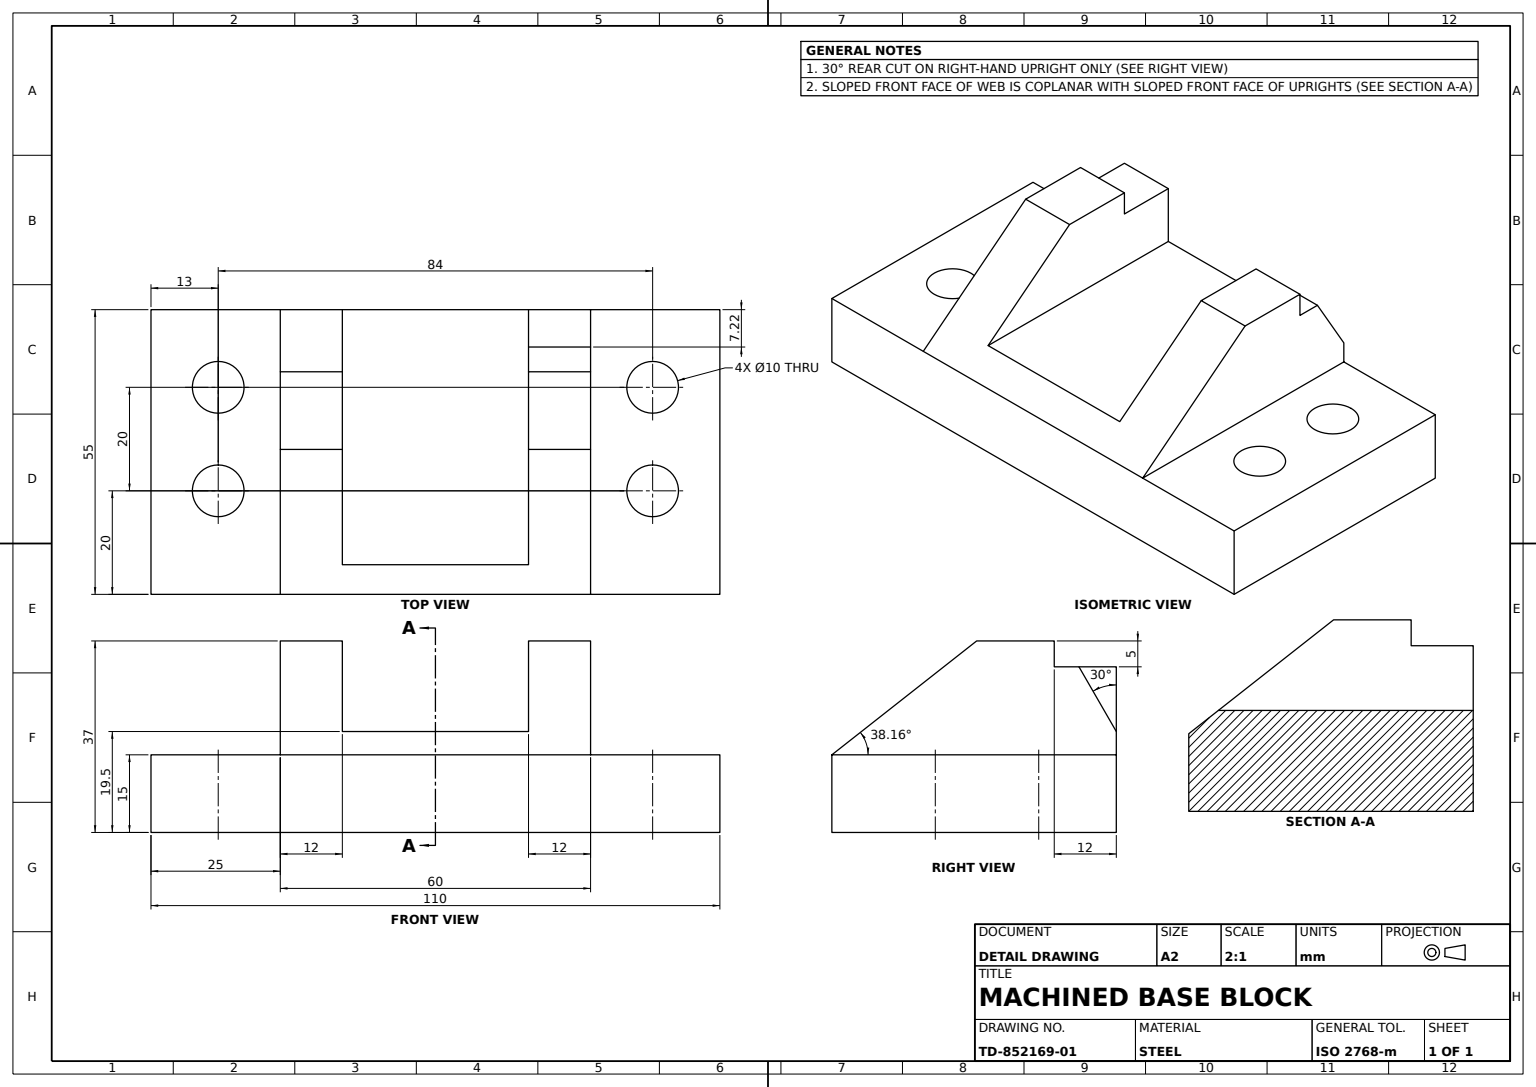
from build123d import *

# Parameters (mm, degrees)
BASE_PLATE_SKETCH_W    = 110
BASE_PLATE_SKETCH_H    = 55
BASE_PLATE_SKETCH_R    = 5
BASE_PLATE_DEPTH       = 15
V_BLOCK_UPRIGHTS_DEPTH = 55
UPRIGHT_NOTCH_SKETCH_W = 12
UPRIGHT_NOTCH_SKETCH_H = 5
UPRIGHT_NOTCH_DEPTH    = 108.791465339
ANGLED_CUT_30DEG_DEPTH = 12


with BuildPart() as part:
    # Base Plate Sketch → Base Plate (new body)
    with BuildSketch(Plane(origin=(0, 0, 0), x_dir=(1, 0, 0), z_dir=(0, 1, 0))):
        with Locations((0, 27.5)):
            Rectangle(BASE_PLATE_SKETCH_W, BASE_PLATE_SKETCH_H)
        with Locations(Location((-42, 40, 0), (0, 0, 270))):
            Circle(BASE_PLATE_SKETCH_R, mode=Mode.SUBTRACT)
        with Locations(Location((-42, 20, 0), (0, 0, 270))):
            Circle(BASE_PLATE_SKETCH_R, mode=Mode.SUBTRACT)
        with Locations(Location((42, 20, 0), (0, 0, 90))):
            Circle(BASE_PLATE_SKETCH_R, mode=Mode.SUBTRACT)
        with Locations(Location((42, 40, 0), (0, 0, 90))):
            Circle(BASE_PLATE_SKETCH_R, mode=Mode.SUBTRACT)
    extrude(amount=BASE_PLATE_DEPTH)

    # V-Block Uprights Sketch → V-Block Uprights (add)
    with BuildSketch(Plane(origin=(0, 0, -55), x_dir=(-1, 0, 0), z_dir=(0, 0, -1))):
        Polygon((-30, 15), (-18, 15), (18, 15), (30, 15), (30, 37), (18, 37), (18, 19.5), (-18, 19.5), (-18, 37), (-30, 37), align=None)
    extrude(amount=-V_BLOCK_UPRIGHTS_DEPTH)

    # Upright Notch Sketch → Upright Notch (cut, through all)
    with BuildSketch(Plane.ZY.offset(30)):
        Polygon((0, 15), (-28, 37), (0, 37), align=None)
        with Locations((-49, 34.5)):
            Rectangle(UPRIGHT_NOTCH_SKETCH_W, UPRIGHT_NOTCH_SKETCH_H)
    extrude(amount=-UPRIGHT_NOTCH_DEPTH, mode=Mode.SUBTRACT)

    # Angled Cut 30deg Sketch → Angled Cut 30deg (cut)
    with BuildSketch(Plane.ZY.offset(-18)):
        Polygon((-55, 19.5), (-47.783121635, 32), (-55, 32), align=None)
    extrude(amount=-ANGLED_CUT_30DEG_DEPTH, mode=Mode.SUBTRACT)


solid = part.part
